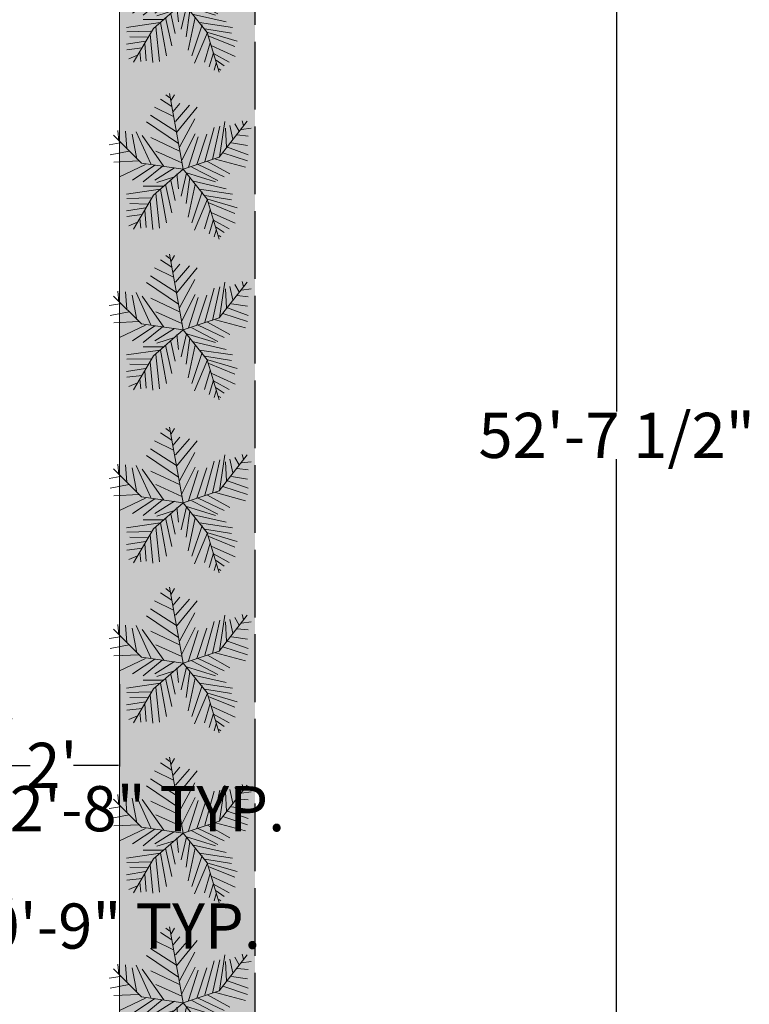
# Model space of a CAD drawing. Units: inches. Extents: x 853 to 1550, y 485 to 1596.
# Tile 11 of 18: x 1420 to 1550, y 1034 to 1208. Entities that reach past the tile are written whole.
import ezdxf

# ---------------------------------------------------------------- set-up
doc = ezdxf.new("R2010")
doc.units = ezdxf.units.IN
doc.header["$MEASUREMENT"] = 0
doc.linetypes.add('ACAD_ISO02W100', pattern=[15, 12, -3])
for name, color, linetype, lineweight in [('A-ANNO-DIMS', 2, 'Continuous', 18), ('C-PROP', 8, 'ACAD_ISO02W100', 25), ('L-PLNT-TREE', 106, 'Continuous', 13), ('lawn', 106, 'Continuous', 18)]:
    doc.layers.add(name, color=color, linetype=linetype, lineweight=lineweight)
doc.layers.add('L-PLNT-PATT', color=85, linetype='Continuous', lineweight=13, true_color=0x58ba48)
doc.styles.get("Standard").update_dxf_attribs({"font": 'arial.ttf'})
doc.dimstyles.get("Standard").update_dxf_attribs({"dimtxt": 8, "dimasz": 0.18, "dimexe": 0.18, "dimexo": 0.0625, "dimgap": 0.09, "dimtad": 0, "dimtih": 1, "dimtoh": 1, "dimzin": 0, "dimdsep": 46, "dimlunit": 3, "dimtxsty": 'Standard', "dimcen": 0.09, "dimadec": 0, "dimazin": 0, "dimtfac": 1, "dimtofl": 0, "dimtmove": 0, "dimatfit": 3, "dimfxl": 1, "dimtolj": 1, "dimtzin": 0, "dimarcsym": 0})

# ---------------------------------------------------------------- blocks, each defined once
blk = doc.blocks.new('*U18')
for p, q in [((-8.737, 47.138), (-17.069, 52.711)), ((-10.186, 53.64), (-13.084, 55.962)), ((0, 0), (-10.5, 57)), ((-9.099, 51.782), (-6.563, 55.962)), ((-7.288, 39.707), (-21.778, 46.673)), ((-7.65, 43.423), (-2.578, 49.46)), ((-5.839, 35.992), (4.667, 48.067)), ((-5.114, 27.632), (10.463, 46.673)), ((-5.114, 28.097), (-24.676, 40.636)), ((-2.941, 16.486), (8.652, 37.85)), ((-3.665, 19.273), (-27.574, 35.527)), ((16.259, 5.805), (23.142, 31.348)), ((22.055, 7.198), (27.489, 32.277)), ((27, 9), (48, 36)), ((27.127, 9.056), (31.112, 35.992)), ((31.836, 30.883), (32.561, 16.486)), ((35.096, 32.741), (37.27, 22.524)), ((38.719, 34.134), (41.979, 28.561)), ((43.791, 29.954), (51.036, 30.883)), ((44.153, 36.456), (45.239, 32.741)), ((-31.5, 4.5), (-52.5, 25.5)), ((-48.585, 21.131), (-49.309, 29.026)), ((-43.513, 28.561), (-42.427, 15.558)), ((-38.442, 26.239), (-34.819, 7.663)), ((-35.544, 28.097), (-24.314, 3.947)), ((-14.533, 2.09), (-30.834, 25.31)), ((-24.314, 23.917), (-2.941, 13.7)), ((-1.129, 6.734), (9.014, 26.704)), ((3.942, 1.625), (11.187, 24.381)), ((10.101, 3.483), (17.708, 26.239)), ((40.53, 25.775), (48.862, 24.846)), ((-47.498, 19.737), (-55.83, 18.344)), ((33.285, 16.486), (48.862, 10.913)), ((36.183, 19.737), (48.137, 17.88)), ((-40.615, 13.7), (-55.105, 10.913)), ((-20.691, 13.7), (-1.129, 4.876)), ((0, 0), (27, 9)), ((24.229, 7.663), (46.688, 1.625)), ((29.662, 12.307), (48.137, 6.269)), ((-33.37, 6.269), (-52.207, 5.34)), ((-28.299, 3.483), (-47.86, -5.805)), ((-21.416, 3.018), (-38.079, -8.128)), ((0, 0), (-31.5, 4.5)), ((-15.982, 2.09), (-30.11, -9.521)), ((0, 0), (-22.5, -19.5)), ((-6.563, 1.161), (-21.416, -8.128)), ((0, 0), (18, -22.5)), ((6.478, 1.625), (26.04, -8.592)), ((11.187, 3.483), (30.749, -5.805)), ((18.07, 5.805), (35.096, -3.483)), ((-6.563, -5.805), (-19.967, -9.985)), ((-4.752, -3.483), (-3.665, -14.629)), ((2.493, -3.019), (-1.491, -20.202)), ((1.769, -2.555), (24.229, -9.521)), ((5.029, -6.27), (2.131, -25.775)), ((-15.257, -12.772), (-30.11, -12.772)), ((-13.446, -11.378), (-8.737, -32.741)), ((-9.461, -8.592), (-6.201, -23.453)), ((9.014, -11.378), (3.58, -35.992)), ((7.565, -9.056), (32.198, -14.629)), ((-17.431, -15.094), (-42.789, -18.809)), ((-24.314, -21.596), (-42.427, -22.06)), ((-22.5, -19.5), (-37.5, -45)), ((-20.691, -18.345), (-17.793, -44.352)), ((-17.069, -15.094), (-12.721, -40.172)), ((14.085, -16.951), (6.478, -40.172)), ((12.274, -15.094), (36.907, -18.809)), ((16.259, -19.738), (36.183, -22.989)), ((-28.299, -29.026), (-42.789, -31.348)), ((-26.849, -26.24), (-40.253, -25.775)), ((-25.038, -23.918), (-22.865, -45.281)), ((18.07, -22.524), (8.289, -45.745)), ((18, -22.5), (27, -52.5)), ((18.433, -22.524), (40.53, -29.026)), ((19.157, -25.311), (38.719, -33.206)), ((-30.834, -34.135), (-42.427, -35.528)), ((-32.646, -36.921), (-31.921, -44.352)), ((-29.023, -30.884), (-27.936, -43.887)), ((20.244, -30.419), (15.897, -44.816)), ((21.331, -32.741), (39.081, -40.636)), ((-34.457, -39.708), (-40.978, -42.494)), ((22.78, -37.85), (19.519, -48.532)), ((22.78, -38.314), (34.372, -44.816)), ((24.591, -43.423), (30.749, -47.603)), ((24.591, -45.745), (23.142, -50.854)), ((26.764, -49.925), (28.213, -50.854))]:
    blk.add_line(p, q)
blk = doc.blocks.new('*D20')
at = {"layer": 'A-ANNO-DIMS', "color": 0, "lineweight": -2, "transparency": 16777216}
for p, q in [((1413.94, 1090.29), (1413.94, 1075.73)), ((1437.94, 1090.29), (1437.94, 1075.73)), ((1414.12, 1075.91), (1422.1, 1075.91)), ((1437.76, 1075.91), (1429.78, 1075.91))]:
    blk.add_line(p, q, dxfattribs=at)
at = {"layer": 'A-ANNO-DIMS', "color": 0, "transparency": 16777216}
for points in [[(1414.12, 1075.94), (1414.12, 1075.88), (1413.94, 1075.91)], [(1437.76, 1075.94), (1437.76, 1075.88), (1437.94, 1075.91)]]:
    blk.add_solid(points, dxfattribs=at)
at = {"layer": 'Defpoints', "color": 0, "transparency": 16777216}
for p in [(1413.94, 1090.36), (1437.94, 1090.36), (1437.94, 1075.91)]:
    blk.add_point(p, dxfattribs=at)
at = {"layer": 'A-ANNO-DIMS', "color": 0, "transparency": 16777216, "insert": (1425.94, 1075.91), "char_height": 8, "attachment_point": 5}
blk.add_mtext("\\A1;2'", dxfattribs=at)
blk = doc.blocks.new('*D53')
at = {"layer": 'A-ANNO-DIMS', "color": 0, "lineweight": -2, "transparency": 16777216}
for p, q in [((1414, 1084.23), (1418.92, 1084.23)), ((1418.74, 1084.05), (1418.74, 1072.46)), ((1418.74, 1052.41), (1418.74, 1064)), ((1414, 1052.23), (1418.92, 1052.23))]:
    blk.add_line(p, q, dxfattribs=at)
at = {"layer": 'A-ANNO-DIMS', "color": 0, "transparency": 16777216}
for points in [[(1418.71, 1084.05), (1418.77, 1084.05), (1418.74, 1084.23)], [(1418.71, 1052.41), (1418.77, 1052.41), (1418.74, 1052.23)]]:
    blk.add_solid(points, dxfattribs=at)
at = {"layer": 'Defpoints', "color": 0, "transparency": 16777216}
for p in [(1413.94, 1084.23), (1418.74, 1084.23), (1413.94, 1052.23)]:
    blk.add_point(p, dxfattribs=at)
at = {"layer": 'A-ANNO-DIMS', "color": 0, "transparency": 16777216, "insert": (1418.74, 1068.23), "char_height": 8, "attachment_point": 5}
blk.add_mtext('\\A1;WINDOW 2\'-8" TYP.', dxfattribs=at)
blk = doc.blocks.new('*D54')
at = {"layer": 'A-ANNO-DIMS', "color": 0, "lineweight": -2, "transparency": 16777216}
for p, q in [((1404.94, 1052.16), (1404.94, 1047.25)), ((1413.94, 1052.16), (1413.94, 1047.25)), ((1405.12, 1047.43), (1413.76, 1047.43)), ((1413.94, 1047.43), (1414.12, 1047.43))]:
    blk.add_line(p, q, dxfattribs=at)
at = {"layer": 'A-ANNO-DIMS', "color": 0, "transparency": 16777216}
for points in [[(1405.12, 1047.46), (1405.12, 1047.4), (1404.94, 1047.43)], [(1413.76, 1047.46), (1413.76, 1047.4), (1413.94, 1047.43)]]:
    blk.add_solid(points, dxfattribs=at)
at = {"layer": 'Defpoints', "color": 0, "transparency": 16777216}
for p in [(1404.94, 1052.23), (1413.94, 1052.23), (1413.94, 1047.43)]:
    blk.add_point(p, dxfattribs=at)
at = {"layer": 'A-ANNO-DIMS', "color": 0, "transparency": 16777216, "insert": (1438.59, 1047.43), "char_height": 8, "attachment_point": 5}
blk.add_mtext('\\A1;0\'-9" TYP.', dxfattribs=at)
blk = doc.blocks.new('*D79')
at = {"layer": 'A-ANNO-DIMS', "color": 0, "lineweight": -2, "transparency": 16777216}
for p, q in [((1438, 1450.13), (1526.24, 1450.13)), ((1526.06, 1449.95), (1526.06, 1138.61)), ((1526.06, 818.81), (1526.06, 1130.15)), ((1438, 818.63), (1526.24, 818.63))]:
    blk.add_line(p, q, dxfattribs=at)
at = {"layer": 'A-ANNO-DIMS', "color": 0, "transparency": 16777216}
for points in [[(1526.03, 1449.95), (1526.09, 1449.95), (1526.06, 1450.13)], [(1526.03, 818.81), (1526.09, 818.81), (1526.06, 818.63)]]:
    blk.add_solid(points, dxfattribs=at)
at = {"layer": 'Defpoints', "color": 0, "transparency": 16777216}
for p in [(1437.94, 1450.13), (1526.06, 1450.13), (1437.94, 818.63)]:
    blk.add_point(p, dxfattribs=at)
at = {"layer": 'A-ANNO-DIMS', "color": 0, "transparency": 16777216, "insert": (1526.06, 1134.38), "char_height": 8, "attachment_point": 5}
blk.add_mtext('\\A1;52\'-7 1/2"', dxfattribs=at)

msp = doc.modelspace()

# ---------------------------------------------------------------- hatches: boundary and pattern name
at = {"layer": 'L-PLNT-PATT'}
h = msp.add_hatch(color=256, dxfattribs=at)
h.dxf.hatch_style = 1
h.paths.add_polyline_path([(1461.937, 1474.129), (933.937, 1474.129), (933.937, 730.129), (933.937, 622.891), (941.686, 622.891), (941.686, 604.895), (957.937, 604.895), (957.937, 1450.129), (1437.937, 1450.129), (1437.937, 604.895), (1454.646, 604.895), (1454.646, 622.891), (1461.937, 622.891), (1461.937, 734.988)])

# ---------------------------------------------------------------- linework, layer by layer
at = {"layer": 'C-PROP'}
msp.add_line((1461.937, 1474.129), (1461.937, 730.129), dxfattribs=at)
at = {"layer": 'lawn'}
msp.add_line((1437.937, 1450.129), (1437.937, 818.629), dxfattribs=at)

# ---------------------------------------------------------------- block references
at = {"layer": 'L-PLNT-TREE', "xscale": 0.2357951711934384, "yscale": 0.2357951711934384, "zscale": 0.2357951711934384}
for p in [(1449.245, 1211.111), (1449.245, 1181.549), (1449.245, 1153.07), (1449.245, 1122.428), (1449.245, 1094.038), (1449.245, 1063.914), (1449.245, 1033.851)]:
    msp.add_blockref('*U18', p, dxfattribs=at)

# ---------------------------------------------------------------- dimensions: what is measured, and where the dimension line sits
at = {"layer": 'A-ANNO-DIMS'}
dim = msp.add_linear_dim(base=(1526.064, 1450.129), p1=(1437.937, 818.629), p2=(1437.937, 1450.129), angle=90, dimstyle='Standard', override={"dimdec": 1, "dimlfac": 1, "dimrnd": 0, "dimzin": 1, "dimdsep": 46, "dimlunit": 4, "dimfrac": 2}, dxfattribs=at)
dim.commit()
dim.dimension.update_dxf_attribs({"geometry": '*D79', "text_midpoint": (1526.064, 1134.379)})
dim = msp.add_linear_dim(base=(1437.937, 1075.913), p1=(1413.937, 1090.357), p2=(1437.937, 1090.357), dimstyle='Standard', override={"dimclrd": 0, "dimclre": 0, "dimclrt": 0}, dxfattribs=at)
dim.commit()
dim.dimension.update_dxf_attribs({"geometry": '*D20', "text_midpoint": (1425.937, 1075.913)})
dim = msp.add_linear_dim(base=(1418.738, 1084.233), p1=(1413.937, 1052.227), p2=(1413.937, 1084.233), angle=90, text='WINDOW <> TYP.', dimstyle='Standard', override={"dimdec": 1, "dimlfac": 1, "dimrnd": 0, "dimzin": 1, "dimdsep": 46, "dimlunit": 4, "dimfrac": 2}, dxfattribs=at)
dim.commit()
dim.dimension.update_dxf_attribs({"geometry": '*D53', "text_midpoint": (1418.738, 1068.23)})
dim = msp.add_linear_dim(base=(1413.937, 1047.426), p1=(1404.937, 1052.227), p2=(1413.937, 1052.227), text='<> TYP.', dimstyle='Standard', override={"dimdec": 1, "dimlfac": 1, "dimrnd": 0, "dimzin": 1, "dimdsep": 46, "dimlunit": 4, "dimfrac": 2}, dxfattribs=at)
dim.commit()
dim.dimension.update_dxf_attribs({"geometry": '*D54', "text_midpoint": (1438.589, 1047.426)})

doc.saveas('drawing.dxf')
